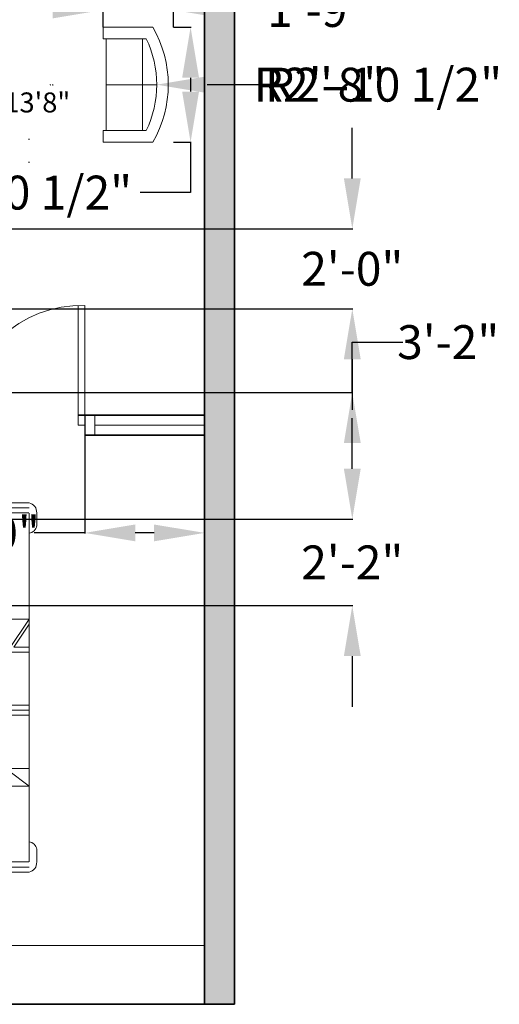
# Model space of a CAD drawing. Units: inches. Extents: x 19 to 15718, y 7 to 930.
# Tile 10 of 11: x 15502 to 15646, y 350 to 646. Entities that reach past the tile are written whole.
import ezdxf

# ---------------------------------------------------------------- set-up
doc = ezdxf.new("R2010")
doc.units = ezdxf.units.IN
doc.header["$MEASUREMENT"] = 0
for name, color, linetype, lineweight in [('A-ANNO-DIMS', 2, 'Continuous', 18), ('A-AREA-IDEN', 7, 'Continuous', 18), ('A-DOOR', 4, 'Continuous', 20), ('A-FLOR', 8, 'Continuous', 18), ('A-FURN', 8, 'Continuous', 18), ('A-GLAZ', 4, 'Continuous', 18), ('A-WALL', 7, 'Continuous', 35), ('C-PKNG-VEHC', 8, 'Continuous', 13)]:
    doc.layers.add(name, color=color, linetype=linetype, lineweight=lineweight)
doc.layers.add('A-WALL-PATT', color=18, linetype='Continuous', lineweight=13, true_color=0x000000)
doc.styles.add('Annotative', font='arial.ttf')
doc.styles.get("Standard").update_dxf_attribs({"font": 'arial.ttf'})
doc.dimstyles.get("Standard").update_dxf_attribs({"dimtxt": 10.18, "dimasz": 15.18, "dimexe": 0.18, "dimexo": 0.0625, "dimgap": 0.09, "dimtad": 0, "dimtih": 1, "dimtoh": 1, "dimdec": 0, "dimzin": 0, "dimdsep": 46, "dimlunit": 3, "dimtxsty": 'Standard', "dimcen": 0.09, "dimadec": 0, "dimazin": 0, "dimtfac": 1, "dimtdec": 0, "dimtofl": 0, "dimtmove": 0, "dimatfit": 3, "dimfxl": 1, "dimtolj": 1, "dimtzin": 0, "dimarcsym": 0})

# ---------------------------------------------------------------- blocks, each defined once
blk = doc.blocks.new('Sofa - Roundback Loveseat 5 ft.')
for p, q in [((0, -32.44198), (0, -5.99998)), ((-24, -33.99998), (-24, -11.46958)), ((-23.9998, -13.38178), (23.99986, -13.38178)), ((24.00004, -33.99998), (24.00004, -11.46958)), ((-24, -32.44198), (24.00004, -32.44198))]:
    blk.add_line(p, q)
for points in [[(-24, -33.99998), (-30, -33.99998), (-30, -7.99998)], [(30.00004, -7.99998), (30.00004, -33.99998), (24.00004, -33.99998)]]:
    blk.add_lwpolyline(points)
for centre, radius, start, end in [((0, -60.24998), 60.24998, 60.13715, 119.8628), ((0, -61.38438), 55.38444, 64.32083, 115.6792)]:
    blk.add_arc(centre, radius, start, end)
blk = doc.blocks.new('*U14')
for p, q in [((5.44, 42.31), (12.12, 42.31)), ((189.69, 42.31), (183.01, 42.31)), ((0.1, -0.41), (0.1, 38.35)), ((2.77, -0.41), (2.77, 38.31)), ((5.44, -0.41), (5.44, 38.24)), ((5.45, 38.31), (16.12, 38.31)), ((16.12, 38.31), (180.34, 38.31)), ((61.52, -0.41), (61.52, 38.31)), ((61.52, 38.31), (77.54, 27.62)), ((64.19, 38.31), (76.2, 30.29)), ((76.2, 30.29), (76.2, 38.31)), ((78.87, 38.31), (78.87, 28.96)), ((106.91, 28.96), (106.91, 38.31)), ((109.58, 27.62), (109.58, 38.31)), ((112.25, 38.31), (112.25, 28.96)), ((140.29, 28.96), (140.29, 38.31)), ((141.62, 27.62), (149.64, 38.31)), ((149.64, -0.41), (149.64, 38.31)), ((189.69, 38.31), (179.01, 38.31)), ((189.69, -0.41), (189.69, 38.24)), ((192.36, -0.41), (192.36, 38.31)), ((195.03, -0.41), (195.03, 38.35)), ((77.54, 27.62), (141.62, 27.62)), ((77.54, -0.41), (77.54, 27.62)), ((78.87, 28.96), (106.91, 28.96)), ((112.25, 28.96), (140.29, 28.96)), ((141.62, -0.41), (141.62, 27.62)), ((5.44, 7.6), (61.52, 15.61)), ((0.1, -0.42), (0.1, -39.18)), ((2.77, -0.41), (2.77, -39.13)), ((5.44, -0.42), (5.44, -39.07)), ((61.52, -0.41), (61.52, -39.13)), ((77.54, -0.41), (77.54, -28.45)), ((141.62, -0.41), (141.62, -28.45)), ((149.64, -0.41), (149.64, -39.13)), ((189.69, -0.42), (189.69, -39.07)), ((192.36, -0.41), (192.36, -39.13)), ((195.03, -0.42), (195.03, -39.18)), ((5.44, -8.42), (61.52, -16.43)), ((61.52, -39.13), (77.54, -28.45)), ((64.19, -39.13), (76.2, -31.12)), ((76.2, -31.12), (76.2, -39.13)), ((77.54, -28.45), (141.62, -28.45)), ((78.87, -39.13), (78.87, -29.79)), ((78.87, -29.79), (106.91, -29.79)), ((106.91, -29.79), (106.91, -39.13)), ((109.58, -28.45), (109.58, -39.13)), ((112.25, -29.79), (140.29, -29.79)), ((112.25, -39.13), (112.25, -29.79)), ((140.29, -29.79), (140.29, -39.13)), ((141.62, -28.45), (149.64, -39.13)), ((5.45, -39.13), (16.12, -39.13)), ((16.12, -39.13), (180.34, -39.13)), ((189.69, -39.13), (179.01, -39.13)), ((5.44, -43.14), (12.12, -43.14)), ((189.69, -43.14), (183.01, -43.14))]:
    blk.add_line(p, q)
for centre, radius, start, end in [((5.06, 37.26), 5.06, 85.6455, 168.0943), ((11.45, 37.64), 4.72, 8.1301, 81.87), ((183.68, 37.64), 4.72, 98.13, 171.8699), ((190.07, 37.26), 5.06, 11.9057, 94.3545), ((5.06, -38.09), 5.06, 191.9057, 274.3545), ((11.45, -38.46), 4.72, 278.13, 351.8699), ((183.68, -38.46), 4.72, 188.1301, 261.87), ((190.07, -38.09), 5.06, 265.6455, 348.0943)]:
    blk.add_arc(centre, radius, start, end)
blk = doc.blocks.new('DOOR-ENTRY-LEAF-36IN')
for p, q in [((0, 6), (0, 39)), ((2, 3), (2, 39)), ((0, 3), (0, 0)), ((2, 3), (0, 3))]:
    blk.add_line(p, q)
blk.add_arc((1, 4), 35.01, 1.6366, 91.6366)
blk = doc.blocks.new('*D72')
at = {"layer": 'A-ANNO-DIMS', "color": 0, "lineweight": -2, "transparency": 16777216}
for p, q in [((15548.36, 643.79), (15553.66, 643.79)), ((15553.48, 628.61), (15553.48, 624.46)), ((15548.36, 609.28), (15553.66, 609.28)), ((15553.48, 609.28), (15553.48, 594.1)), ((15553.48, 594.1), (15538.3, 594.1))]:
    blk.add_line(p, q, dxfattribs=at)
at = {"layer": 'A-ANNO-DIMS', "color": 0, "transparency": 16777216}
for points in [[(15550.95, 628.61), (15556.01, 628.61), (15553.48, 643.79)], [(15550.95, 624.46), (15556.01, 624.46), (15553.48, 609.28)]]:
    blk.add_solid(points, dxfattribs=at)
at = {"layer": 'Defpoints', "color": 0, "transparency": 16777216}
for p in [(15548.3, 643.79), (15548.3, 609.28), (15553.48, 609.28)]:
    blk.add_point(p, dxfattribs=at)
at = {"layer": 'A-ANNO-DIMS', "color": 0, "transparency": 16777216, "insert": (15469.57, 594.1), "char_height": 10.18, "attachment_point": 5}
blk.add_mtext('\\A1;LOVESEAT 2\'-10 1/2"', dxfattribs=at)
blk = doc.blocks.new('*D73')
at = {"layer": 'A-ANNO-DIMS', "color": 0, "lineweight": -2, "transparency": 16777216}
for p, q in [((15512.03, 648.97), (15496.85, 648.97)), ((15527.21, 643.85), (15527.21, 649.15)), ((15548.3, 643.85), (15548.3, 649.15)), ((15563.48, 648.97), (15578.66, 648.97))]:
    blk.add_line(p, q, dxfattribs=at)
at = {"layer": 'A-ANNO-DIMS', "color": 0, "transparency": 16777216}
for points in [[(15512.03, 651.5), (15512.03, 646.44), (15527.21, 648.97)], [(15563.48, 651.5), (15563.48, 646.44), (15548.3, 648.97)]]:
    blk.add_solid(points, dxfattribs=at)
at = {"layer": 'Defpoints', "color": 0, "transparency": 16777216}
for p in [(15548.3, 648.97), (15527.21, 643.79), (15548.3, 643.79)]:
    blk.add_point(p, dxfattribs=at)
at = {"layer": 'A-ANNO-DIMS', "color": 0, "transparency": 16777216, "insert": (15591.8, 648.97), "char_height": 10.18, "attachment_point": 5}
blk.add_mtext('\\A1;1\'-9"', dxfattribs=at)
blk = doc.blocks.new('*D79')
at = {"layer": 'A-ANNO-DIMS', "color": 0, "lineweight": -2, "transparency": 16777216}
for p, q in [((15602.03, 534), (15602.03, 549.18)), ((15602.03, 549.18), (15617.21, 549.18)), ((15082.89, 534), (15602.21, 534)), ((15602.03, 511.14), (15602.03, 518.82)), ((15082.89, 495.96), (15602.21, 495.96))]:
    blk.add_line(p, q, dxfattribs=at)
at = {"layer": 'A-ANNO-DIMS', "color": 0, "transparency": 16777216}
for points in [[(15599.5, 518.82), (15604.56, 518.82), (15602.03, 534)], [(15599.5, 511.14), (15604.56, 511.14), (15602.03, 495.96)]]:
    blk.add_solid(points, dxfattribs=at)
at = {"layer": 'Defpoints', "color": 0, "transparency": 16777216}
for p in [(15082.83, 534), (15602.03, 534), (15082.83, 495.96)]:
    blk.add_point(p, dxfattribs=at)
at = {"layer": 'A-ANNO-DIMS', "color": 0, "transparency": 16777216, "insert": (15630.83, 549.18), "char_height": 10.18, "attachment_point": 5}
blk.add_mtext('\\A1;3\'-2"', dxfattribs=at)
blk = doc.blocks.new('*D80')
at = {"layer": 'A-ANNO-DIMS', "color": 0, "lineweight": -2, "transparency": 16777216}
for p, q in [((15602.030581, 511.142303), (15602.030581, 526.322303)), ((15181.899116, 495.962303), (15602.210581, 495.962303)), ((15181.899116, 469.995573), (15602.210581, 469.995573)), ((15602.030581, 454.815573), (15602.030581, 439.635573))]:
    blk.add_line(p, q, dxfattribs=at)
at = {"layer": 'A-ANNO-DIMS', "color": 0, "transparency": 16777216}
for points in [[(15599.500581, 511.142303), (15604.560581, 511.142303), (15602.030581, 495.962303)], [(15599.500581, 454.815573), (15604.560581, 454.815573), (15602.030581, 469.995573)]]:
    blk.add_solid(points, dxfattribs=at)
at = {"layer": 'Defpoints', "color": 0, "transparency": 16777216}
for p in [(15181.836616, 495.962303), (15602.030581, 495.962303), (15181.836616, 469.995573)]:
    blk.add_point(p, dxfattribs=at)
at = {"layer": 'A-ANNO-DIMS', "color": 0, "transparency": 16777216, "insert": (15602.030581, 482.978938), "char_height": 10.18, "attachment_point": 5}
blk.add_mtext('\\A1;2\'-2"', dxfattribs=at)
blk = doc.blocks.new('*D82')
at = {"layer": 'A-ANNO-DIMS', "color": 0, "lineweight": -2, "transparency": 16777216}
for p, q in [((15602.030581, 598.383955), (15602.030581, 613.563955)), ((15377.073779, 583.203955), (15602.210581, 583.203955)), ((15377.073779, 559.203955), (15602.210581, 559.203955)), ((15602.030581, 544.023955), (15602.030581, 528.843955))]:
    blk.add_line(p, q, dxfattribs=at)
at = {"layer": 'A-ANNO-DIMS', "color": 0, "transparency": 16777216}
for points in [[(15599.500581, 598.383955), (15604.560581, 598.383955), (15602.030581, 583.203955)], [(15599.500581, 544.023955), (15604.560581, 544.023955), (15602.030581, 559.203955)]]:
    blk.add_solid(points, dxfattribs=at)
at = {"layer": 'Defpoints', "color": 0, "transparency": 16777216}
for p in [(15377.011279, 583.203955), (15602.030581, 583.203955), (15377.011279, 559.203955)]:
    blk.add_point(p, dxfattribs=at)
at = {"layer": 'A-ANNO-DIMS', "color": 0, "transparency": 16777216, "insert": (15602.030581, 571.203955), "char_height": 10.18, "attachment_point": 5}
blk.add_mtext('\\A1;2\'-0"', dxfattribs=at)
blk = doc.blocks.new('*D85')
at = {"layer": 'A-ANNO-DIMS', "color": 0, "lineweight": -2, "transparency": 16777216}
for p, q in [((15521.68, 527.14), (15521.68, 491.67)), ((15557.68, 527.14), (15557.68, 491.67)), ((15521.68, 491.85), (15506.5, 491.85)), ((15542.5, 491.85), (15536.86, 491.85))]:
    blk.add_line(p, q, dxfattribs=at)
at = {"layer": 'A-ANNO-DIMS', "color": 0, "transparency": 16777216}
for points in [[(15536.86, 494.38), (15536.86, 489.32), (15521.68, 491.85)], [(15542.5, 494.38), (15542.5, 489.32), (15557.68, 491.85)]]:
    blk.add_solid(points, dxfattribs=at)
at = {"layer": 'Defpoints', "color": 0, "transparency": 16777216}
for p in [(15521.68, 527.2), (15557.68, 527.2), (15521.68, 491.85)]:
    blk.add_point(p, dxfattribs=at)
at = {"layer": 'A-ANNO-DIMS', "color": 0, "transparency": 16777216, "insert": (15492.88, 491.85), "char_height": 10.18, "attachment_point": 5}
blk.add_mtext('\\A1;3\'-0"', dxfattribs=at)
blk = doc.blocks.new('*D90')
at = {"layer": 'A-ANNO-DIMS', "color": 0, "lineweight": -2, "transparency": 16777216}
for p, q in [((15520.15, 706.74), (15504.97, 706.74)), ((15504.97, 706.74), (15504.97, 683.11)), ((15504.88, 603.26), (15505.06, 603.26)), ((15504.97, 603.17), (15504.97, 603.35))]:
    blk.add_line(p, q, dxfattribs=at)
at = {"layer": 'A-ANNO-DIMS', "color": 0, "transparency": 16777216}
blk.add_solid([(15502.44, 683.11), (15507.5, 683.11), (15504.97, 667.93)], dxfattribs=at)
at = {"layer": 'Defpoints', "color": 0, "transparency": 16777216}
for p in [(15504.97, 667.93), (15504.97, 603.26)]:
    blk.add_point(p, dxfattribs=at)
at = {"layer": 'A-ANNO-DIMS', "color": 0, "transparency": 16777216, "insert": (15550.51, 706.74), "char_height": 10.18, "attachment_point": 5}
blk.add_mtext('\\A1;R5\'-4 1/2"', dxfattribs=at)
blk = doc.blocks.new('*D91')
at = {"layer": 'A-ANNO-DIMS', "color": 0, "lineweight": -2, "transparency": 16777216}
for p, q in [((15520.15, 707.71), (15504.97, 707.71)), ((15504.97, 707.71), (15504.97, 686.31)), ((15504.88, 610.17), (15505.06, 610.17)), ((15504.97, 610.08), (15504.97, 610.26))]:
    blk.add_line(p, q, dxfattribs=at)
at = {"layer": 'A-ANNO-DIMS', "color": 0, "transparency": 16777216}
blk.add_solid([(15502.44, 686.31), (15507.5, 686.31), (15504.97, 671.13)], dxfattribs=at)
at = {"layer": 'Defpoints', "color": 0, "transparency": 16777216}
for p in [(15504.97, 671.13), (15504.97, 610.17)]:
    blk.add_point(p, dxfattribs=at)
at = {"layer": 'A-ANNO-DIMS', "color": 0, "transparency": 16777216, "insert": (15538.64, 707.71), "char_height": 10.18, "attachment_point": 5}
blk.add_mtext('\\A1;R5\'-1"', dxfattribs=at)
blk = doc.blocks.new('*D92')
at = {"layer": 'A-ANNO-DIMS', "color": 0, "lineweight": -2, "transparency": 16777216}
for p, q in [((15512.02, 626.53), (15512.2, 626.53)), ((15512.11, 626.44), (15512.11, 626.62)), ((15577.13, 626.53), (15561.95, 626.53))]:
    blk.add_line(p, q, dxfattribs=at)
at = {"layer": 'A-ANNO-DIMS', "color": 0, "transparency": 16777216}
blk.add_solid([(15561.95, 629.06), (15561.95, 624), (15546.77, 626.53)], dxfattribs=at)
at = {"layer": 'Defpoints', "color": 0, "transparency": 16777216}
for p in [(15512.11, 626.53), (15546.77, 626.53)]:
    blk.add_point(p, dxfattribs=at)
at = {"layer": 'A-ANNO-DIMS', "color": 0, "transparency": 16777216, "insert": (15611.43, 626.53), "char_height": 10.18, "attachment_point": 5}
blk.add_mtext('\\A1;R2\'-10 1/2"', dxfattribs=at)
blk = doc.blocks.new('*D93')
at = {"layer": 'A-ANNO-DIMS', "color": 0, "lineweight": -2, "transparency": 16777216}
for p, q in [((15511.37, 626.53), (15511.55, 626.53)), ((15511.46, 626.44), (15511.46, 626.62)), ((15573.67, 626.53), (15558.49, 626.53))]:
    blk.add_line(p, q, dxfattribs=at)
at = {"layer": 'A-ANNO-DIMS', "color": 0, "transparency": 16777216}
blk.add_solid([(15558.49, 629.06), (15558.49, 624), (15543.31, 626.53)], dxfattribs=at)
at = {"layer": 'Defpoints', "color": 0, "transparency": 16777216}
for p in [(15511.46, 626.53), (15543.31, 626.53)]:
    blk.add_point(p, dxfattribs=at)
at = {"layer": 'A-ANNO-DIMS', "color": 0, "transparency": 16777216, "insert": (15592.17, 626.53), "char_height": 10.18, "attachment_point": 5}
blk.add_mtext('\\A1;R2\'-8"', dxfattribs=at)

msp = doc.modelspace()

# ---------------------------------------------------------------- hatches: boundary and pattern name
at = {"layer": 'A-WALL-PATT'}
h = msp.add_hatch(color=256, dxfattribs=at)
h.dxf.hatch_style = 1
h.paths.add_polyline_path([(15566.68, 830.2), (15266.68, 830.2), (15266.68, 629.2), (15275.68, 629.2), (15275.68, 641.2), (15301.68, 641.2), (15301.68, 589.2), (15275.68, 589.2), (15275.68, 601.2), (15266.68, 601.2), (15266.68, 350.2), (15275.68, 350.2), (15275.68, 359.2), (15275.68, 457.2), (15413.68, 457.2), (15413.68, 471.04), (15407.68, 471.04), (15407.68, 463.2), (15275.68, 463.2), (15275.68, 583.59), (15276.07, 583.2), (15276.65, 583.2), (15277.42, 583.97), (15276.36, 585.03), (15279.54, 588.22), (15280.6, 587.16), (15281.66, 588.22), (15282.72, 587.16), (15283.78, 588.22), (15284.85, 587.16), (15285.91, 588.22), (15286.97, 587.16), (15288.03, 588.22), (15289.09, 587.16), (15290.15, 588.22), (15291.21, 587.16), (15292.27, 588.22), (15293.33, 587.16), (15294.39, 588.22), (15295.45, 587.16), (15296.51, 588.22), (15297.57, 587.16), (15298.63, 588.22), (15299.69, 587.16), (15300.76, 588.22), (15301.82, 587.16), (15302.88, 588.22), (15303.94, 587.16), (15305, 588.22), (15306.06, 587.16), (15307.68, 588.78), (15307.68, 641.2), (15407.68, 641.2), (15413.68, 641.2), (15413.68, 647.2), (15407.68, 647.2), (15275.68, 647.2), (15275.68, 767.2), (15336.68, 767.2), (15336.68, 773.2), (15275.68, 773.2), (15275.68, 821.2), (15375.68, 821.2), (15381.68, 821.2), (15407.68, 821.2), (15413.68, 821.2), (15557.68, 821.2), (15557.68, 697.2), (15452.68, 697.2), (15452.68, 696.2, -0.014283), (15452.68, 694.2), (15452.68, 691.2), (15557.68, 691.2), (15557.68, 527.2), (15557.68, 521.2), (15557.68, 359.2), (15557.68, 350.2), (15566.68, 350.2)])
h.paths.add_polyline_path([(15416.63, 527.2), (15413.68, 527.2), (15407.68, 527.2), (15407.68, 521.04), (15413.68, 521.04), (15413.68, 521.2), (15416.63, 521.2)], flags=17)
h.paths.add_polyline_path([(15432.13, 393.97), (15308.13, 393.97), (15308.13, 425.59), (15299.13, 425.59), (15299.13, 384.97), (15432.13, 384.97)], flags=17)
h.paths.add_polyline_path([(15308.13, 457.2), (15299.13, 457.2), (15299.13, 425.59), (15308.13, 425.59)], flags=17)
h.paths.add_polyline_path([(15425.57, 359.2), (15275.68, 359.2), (15275.68, 350.2), (15425.57, 350.2)], flags=17)
h.paths.add_polyline_path([(15413.68, 797.2), (15407.68, 797.2), (15407.68, 773.2), (15381.68, 773.2), (15381.68, 797.2), (15375.68, 797.2), (15375.68, 773.2), (15375.68, 767.2), (15407.68, 767.2), (15407.68, 686.2), (15408.68, 686.2, -0.014283), (15410.68, 686.2), (15413.68, 686.2), (15413.68, 691.2), (15413.68, 697.2)], flags=17)
h.paths.add_polyline_path([(15413.68, 608.2), (15410.68, 608.2, -0.017236), (15408.68, 608.2), (15407.68, 608.2), (15407.68, 589.2), (15388.16, 589.2, -0.313626), (15386.75, 588.23), (15381.37, 588.23), (15380.3, 587.16), (15381.37, 586.1), (15380.3, 585.03), (15382.14, 583.2), (15407.68, 583.2), (15413.68, 583.2)], flags=17)

# ---------------------------------------------------------------- linework, layer by layer
at = {"layer": 'A-DOOR'}
msp.add_line((15524.68, 521.2), (15524.68, 527.2), dxfattribs=at)
at = {"layer": 'A-FLOR'}
msp.add_line((15557.68, 367.9), (15424.65, 367.9), dxfattribs=at)
at = {"layer": 'A-GLAZ'}
msp.add_line((15524.68, 524.2), (15557.68, 524.2), dxfattribs=at)
at = {"layer": 'A-WALL'}
for p, q in [((15566.68, 830.2), (15566.68, 350.2)), ((15557.68, 691.2), (15557.68, 527.2)), ((15519.68, 527.2), (15557.68, 527.2)), ((15557.68, 521.2), (15557.68, 527.2)), ((15521.68, 521.2), (15557.68, 521.2)), ((15557.68, 521.2), (15557.68, 359.2)), ((15557.68, 359.2), (15557.68, 350.2)), ((15425.57, 350.2), (15557.68, 350.2)), ((15566.68, 350.2), (15557.68, 350.2))]:
    msp.add_line(p, q, dxfattribs=at)

# ---------------------------------------------------------------- block references
at = {"layer": 'A-DOOR', "extrusion": (0, 0, -1), "zscale": -1}
msp.add_blockref('DOOR-ENTRY-LEAF-36IN', (-15521.68, 521.2), dxfattribs=at)
at = {"layer": 'A-FURN', "xscale": 0.575231885967034, "yscale": 0.575231885967034, "zscale": 0.575231885967034, "rotation": 270}
msp.add_blockref('Sofa - Roundback Loveseat 5 ft.', (15546.77, 626.53), dxfattribs=at)
at = {"layer": 'C-PKNG-VEHC', "xscale": 0.5691226359303588, "yscale": 0.5691226359303588, "zscale": 0.5691226359303588, "rotation": 270}
msp.add_blockref('*U14', (15483.19, 500.93), dxfattribs=at)

# ---------------------------------------------------------------- texts
at = {"layer": 'A-AREA-IDEN', "insert": (15473.71, 634.19), "char_height": 6, "width": 68.1983, "attachment_point": 1, "style": 'Annotative'}
msp.add_mtext('living\\P12\'4"x13\'8"', dxfattribs=at)

# ---------------------------------------------------------------- dimensions: what is measured, and where the dimension line sits
at = {"layer": 'A-ANNO-DIMS'}
for center, mpoint, picture, middle in [((15504.97, 603.26), (15504.97, 667.93), '*D90', (15550.51, 706.74)), ((15504.97, 610.17), (15504.97, 671.13), '*D91', (15538.64, 707.71))]:
    dim = msp.add_radius_dim(center=center, mpoint=mpoint, dimstyle='Standard', override={"dimdec": 1, "dimlfac": 1, "dimrnd": 0, "dimzin": 1, "dimdsep": 46, "dimlunit": 4, "dimfrac": 2}, dxfattribs=at)
    dim.commit()
    dim.dimension.update_dxf_attribs({"geometry": picture, "text_midpoint": middle, "dimtype": 164})
dim = msp.add_linear_dim(base=(15548.3, 648.97), p1=(15527.21, 643.79), p2=(15548.3, 643.79), dimstyle='Standard', override={"dimdec": 1, "dimlfac": 1, "dimrnd": 0, "dimzin": 1, "dimdsep": 46, "dimlunit": 4, "dimfrac": 2}, dxfattribs=at)
dim.commit()
dim.dimension.update_dxf_attribs({"geometry": '*D73', "text_midpoint": (15591.8, 648.97)})
dim = msp.add_linear_dim(base=(15553.48, 609.28), p1=(15548.3, 643.79), p2=(15548.3, 609.28), angle=270, text='LOVESEAT <>', dimstyle='Standard', override={"dimdec": 1, "dimlfac": 1, "dimrnd": 0, "dimzin": 1, "dimdsep": 46, "dimlunit": 4, "dimfrac": 2}, dxfattribs=at)
dim.commit()
dim.dimension.update_dxf_attribs({"geometry": '*D72', "text_midpoint": (15469.57, 594.1)})
for center, mpoint, picture, middle in [((15512.11, 626.53), (15546.77, 626.53), '*D92', (15611.43, 626.53)), ((15511.4553, 626.534), (15543.3142, 626.534), '*D93', (15592.166, 626.534))]:
    dim = msp.add_radius_dim(center=center, mpoint=mpoint, dimstyle='Standard', override={"dimdec": 1, "dimlfac": 1, "dimrnd": 0, "dimzin": 1, "dimdsep": 46, "dimlunit": 4, "dimfrac": 2}, dxfattribs=at)
    dim.commit()
    dim.dimension.update_dxf_attribs({"geometry": picture, "text_midpoint": middle})
for base, p1, p2, angle, picture, middle in [((15602.03, 583.2), (15377.01, 559.2), (15377.01, 583.2), 90, '*D82', (15602.03, 571.2)), ((15602.03, 534), (15082.83, 495.96), (15082.83, 534), 90, '*D79', (15630.83, 549.18)), ((15521.68, 491.85), (15557.68, 527.2), (15521.68, 527.2), 180, '*D85', (15492.88, 491.85)), ((15602.03, 495.96), (15181.84, 470), (15181.84, 495.96), 90, '*D80', (15602.03, 482.98))]:
    dim = msp.add_linear_dim(base=base, p1=p1, p2=p2, angle=angle, dimstyle='Standard', override={"dimdec": 1, "dimlfac": 1, "dimrnd": 0, "dimzin": 1, "dimdsep": 46, "dimlunit": 4, "dimfrac": 2}, dxfattribs=at)
    dim.commit()
    dim.dimension.update_dxf_attribs({"geometry": picture, "text_midpoint": middle})

doc.saveas('drawing.dxf')
